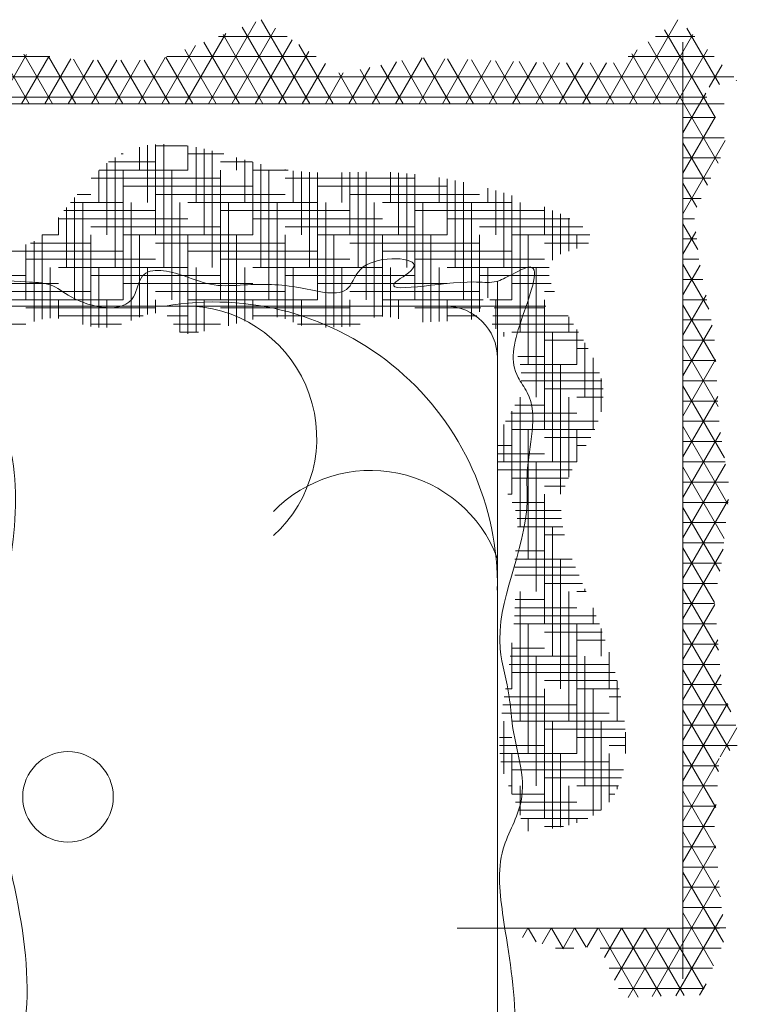
# Model space of a CAD drawing. Units: inches. Extents: x 3731 to 4318, y 1310 to 2388.
# Tile 38 of 57: x 3897 to 3942, y 2243 to 2305. Entities that reach past the tile are written whole.
import ezdxf

# ---------------------------------------------------------------- set-up
doc = ezdxf.new("R2010")
doc.units = ezdxf.units.IN
doc.layers.add('A-FURN', color=8, linetype='Continuous', lineweight=13)

# ---------------------------------------------------------------- blocks, each defined once
blk = doc.blocks.new('A$C200C7901')
for p, q in [((2.3121, 1.6596), (2.3121, 0.0201)), ((2, 0.2957), (2, 1.2957)), ((2.0224, 0.9977), (2.0224, 1.1977)), ((2.0224, 0.9977), (2.0224, 1.1977)), ((1.9974, 0.5977), (1.9974, 0.7977)), ((1.9974, 0.5977), (1.9974, 0.7977)), ((2.0724, 0.5977), (2.0724, 0.7977)), ((2.0724, 0.5977), (2.0724, 0.7977)), ((2.1474, 0.5977), (2.1474, 0.7977)), ((2.1474, 0.5977), (2.1474, 0.7977)), ((1.9849, 0.5477), (1.9849, 0.7477)), ((1.9849, 0.5477), (1.9849, 0.7477)), ((2.0599, 0.5477), (2.0599, 0.7477)), ((2.0599, 0.5477), (2.0599, 0.7477)), ((2.1349, 0.5477), (2.1349, 0.7477)), ((2.1349, 0.5477), (2.1349, 0.7477)), ((1.0407, 0.0275), (1.0407, 0.4323)), ((0.4061, 0.3703), (2.0386, 0.3703)), ((2.4073, 0.0839), (0.9625, 0.0839))]:
    blk.add_line(p, q)
at = {"linetype": 'ByBlock'}
for p, q in [((2.3224, 0.0468), (2.3224, 1.6627)), ((2.3224, 0.0468), (2.3224, 1.6627)), ((2.3537, 0.0056), (2.3537, 1.634)), ((2.3537, 0.0056), (2.3537, 1.634)), ((1.9724, 1.0977), (1.9724, 1.2927)), ((1.9724, 1.0977), (1.9724, 1.2927)), ((2.0474, 1.0977), (2.0474, 1.2977)), ((2.0474, 1.0977), (2.0474, 1.2977)), ((2.3849, 1.0607), (2.3849, 1.3013)), ((2.3849, 1.0607), (2.3849, 1.3013)), ((2.0349, 1.0477), (2.0349, 1.2477)), ((2.0349, 1.0477), (2.0349, 1.2477)), ((2.0099, 0.9477), (2.0099, 1.1477)), ((2.0099, 0.9477), (2.0099, 1.1477)), ((2.0849, 0.9477), (2.0849, 1.1477)), ((2.0849, 0.9477), (2.0849, 1.1477)), ((2.3121, 1.1408), (2.3884, 1.0967)), ((2.3121, 1.1408), (2.3884, 1.0967)), ((2.3121, 1.0928), (2.3915, 1.1386)), ((2.3121, 1.0928), (2.3915, 1.1386)), ((1.9974, 0.8977), (1.9974, 1.0977)), ((1.9974, 0.8977), (1.9974, 1.0977)), ((2.0099, 1.0977), (2.095, 1.0977)), ((2.0099, 1.0977), (2.095, 1.0977)), ((2.0724, 0.8977), (2.0724, 1.0977)), ((2.0724, 0.8977), (2.0724, 1.0977)), ((2.3121, 1.1047), (2.3851, 1.0625)), ((2.3121, 1.1047), (2.3851, 1.0625)), ((2.3121, 1.0567), (2.3887, 1.1009)), ((2.3121, 1.0567), (2.3887, 1.1009)), ((1.9763, 1.0852), (2.1005, 1.0852)), ((1.9763, 1.0852), (2.1005, 1.0852)), ((2.0974, 0.9977), (2.0974, 1.0909)), ((2.0974, 0.9977), (2.0974, 1.0909)), ((1.9799, 1.0727), (2.1099, 1.0727)), ((1.9799, 1.0727), (2.1099, 1.0727)), ((2.1099, 1.0477), (2.1099, 1.0729)), ((2.1099, 1.0477), (2.1099, 1.0729)), ((2.3121, 1.0686), (2.3813, 1.0286)), ((2.3121, 1.0686), (2.3813, 1.0286)), ((1.9815, 1.0602), (2.0599, 1.0602)), ((1.9815, 1.0602), (2.0599, 1.0602)), ((2.3121, 1.0206), (2.3851, 1.0628)), ((2.3121, 1.0206), (2.3851, 1.0628)), ((1.981, 1.0477), (2.0099, 1.0477)), ((1.981, 1.0477), (2.0099, 1.0477)), ((1.9849, 0.9171), (1.9849, 1.0477)), ((1.9849, 0.9171), (1.9849, 1.0477)), ((2.0599, 0.8477), (2.0599, 1.0477)), ((2.0599, 0.8477), (2.0599, 1.0477)), ((2.0599, 1.0352), (2.1523, 1.0352)), ((2.0599, 1.0352), (2.1523, 1.0352)), ((2.1099, 1.0477), (2.137, 1.0477)), ((2.1099, 1.0477), (2.137, 1.0477)), ((2.1349, 0.8477), (2.1349, 1.0477)), ((2.1349, 0.8477), (2.1349, 1.0477)), ((2.1474, 0.8977), (2.1474, 1.0391)), ((2.1474, 0.8977), (2.1474, 1.0391)), ((2.0099, 1.0227), (2.1678, 1.0227)), ((2.0099, 1.0227), (2.1678, 1.0227)), ((2.1599, 0.9477), (2.1599, 1.029)), ((2.1599, 0.9477), (2.1599, 1.029)), ((2.1724, 0.9977), (2.1724, 1.0189)), ((2.1724, 0.9977), (2.1724, 1.0189)), ((2.3121, 1.0325), (2.3795, 0.9936)), ((2.3121, 1.0325), (2.3795, 0.9936)), ((2.3121, 0.9846), (2.3809, 1.0242)), ((2.3121, 0.9846), (2.3809, 1.0242)), ((1.9718, 1.0102), (2.1599, 1.0102)), ((1.9718, 1.0102), (2.1599, 1.0102)), ((1.9688, 0.9977), (2.1099, 0.9977)), ((1.9688, 0.9977), (2.1099, 0.9977)), ((1.9724, 0.9504), (1.9724, 0.9977)), ((1.9724, 0.9504), (1.9724, 0.9977)), ((2.0474, 0.7977), (2.0474, 0.9977)), ((2.0474, 0.7977), (2.0474, 0.9977)), ((2.1224, 0.7977), (2.1224, 0.9977)), ((2.1224, 0.7977), (2.1224, 0.9977)), ((2.1974, 0.7977), (2.1974, 0.9972)), ((2.1974, 0.7977), (2.1974, 0.9972)), ((2.3121, 0.9964), (2.3795, 0.9575)), ((2.3121, 0.9964), (2.3795, 0.9575)), ((2.3121, 0.9485), (2.3795, 0.9874)), ((2.3121, 0.9485), (2.3795, 0.9874)), ((1.9671, 0.9852), (2.0599, 0.9852)), ((1.9671, 0.9852), (2.0599, 0.9852)), ((1.9672, 0.9727), (2.0099, 0.9727)), ((1.9672, 0.9727), (2.0099, 0.9727)), ((2.1099, 0.9727), (2.2204, 0.9727)), ((2.1099, 0.9727), (2.2204, 0.9727)), ((2.1599, 0.9852), (2.2095, 0.9852)), ((2.1599, 0.9852), (2.2095, 0.9852)), ((2.2099, 0.8477), (2.2099, 0.9848)), ((2.2099, 0.8477), (2.2099, 0.9848)), ((2.0599, 0.9602), (2.2294, 0.9602)), ((2.0599, 0.9602), (2.2294, 0.9602)), ((2.2224, 0.8977), (2.2224, 0.9702)), ((2.2224, 0.8977), (2.2224, 0.9702)), ((2.3121, 0.9603), (2.3795, 0.9215)), ((2.3121, 0.9603), (2.3795, 0.9215)), ((2.0099, 0.9477), (2.2099, 0.9477)), ((2.0099, 0.9477), (2.2099, 0.9477)), ((2.0349, 0.7477), (2.0349, 0.9477)), ((2.0349, 0.7477), (2.0349, 0.9477)), ((2.1099, 0.7477), (2.1099, 0.9477)), ((2.1099, 0.7477), (2.1099, 0.9477)), ((2.1849, 0.7477), (2.1849, 0.9477)), ((2.1849, 0.7477), (2.1849, 0.9477)), ((2.2349, 0.9477), (2.2349, 0.9506)), ((2.2349, 0.9477), (2.2349, 0.9506)), ((2.3121, 0.9124), (2.3795, 0.9513)), ((2.3121, 0.9124), (2.3795, 0.9513)), ((1.9781, 0.9352), (2.1599, 0.9352)), ((1.9781, 0.9352), (2.1599, 0.9352)), ((1.9829, 0.9227), (2.1099, 0.9227)), ((1.9829, 0.9227), (2.1099, 0.9227)), ((2.2099, 0.9227), (2.2455, 0.9227)), ((2.2099, 0.9227), (2.2455, 0.9227)), ((2.3121, 0.9243), (2.3838, 0.8829)), ((2.3121, 0.9243), (2.3838, 0.8829)), ((2.3121, 0.8763), (2.3795, 0.9152)), ((2.3121, 0.8763), (2.3795, 0.9152)), ((1.9871, 0.9102), (2.0599, 0.9102)), ((1.9871, 0.9102), (2.0599, 0.9102)), ((1.9894, 0.8977), (2.0099, 0.8977)), ((1.9894, 0.8977), (2.0099, 0.8977)), ((2.0224, 0.6977), (2.0224, 0.8977)), ((2.0224, 0.6977), (2.0224, 0.8977)), ((2.0974, 0.6977), (2.0974, 0.8977)), ((2.0974, 0.6977), (2.0974, 0.8977)), ((2.1099, 0.8977), (2.2496, 0.8977)), ((2.1099, 0.8977), (2.2496, 0.8977)), ((2.1599, 0.9102), (2.2481, 0.9102)), ((2.1599, 0.9102), (2.2481, 0.9102)), ((2.1724, 0.6977), (2.1724, 0.8977)), ((2.1724, 0.6977), (2.1724, 0.8977)), ((2.2474, 0.8489), (2.2474, 0.8977)), ((2.2474, 0.8489), (2.2474, 0.8977)), ((2.0599, 0.8852), (2.2501, 0.8852)), ((2.0599, 0.8852), (2.2501, 0.8852)), ((2.3121, 0.8882), (2.4022, 0.8362)), ((2.3121, 0.8882), (2.4022, 0.8362)), ((2.3121, 0.8402), (2.3842, 0.8818)), ((2.3121, 0.8402), (2.3842, 0.8818)), ((1.9724, 0.7977), (1.9724, 0.8703)), ((1.9724, 0.7977), (1.9724, 0.8703)), ((1.9849, 0.8477), (1.9849, 0.88)), ((1.9849, 0.8477), (1.9849, 0.88)), ((2.0099, 0.8727), (2.2099, 0.8727)), ((2.0099, 0.8727), (2.2099, 0.8727)), ((2.3849, 0.6497), (2.3849, 0.8801)), ((2.3849, 0.6497), (2.3849, 0.8801)), ((1.9599, 0.8317), (1.9599, 0.8604)), ((1.9599, 0.8317), (1.9599, 0.8604)), ((1.9599, 0.8602), (2.1599, 0.8602)), ((1.9599, 0.8602), (2.1599, 0.8602)), ((2.3121, 0.8041), (2.3958, 0.8524)), ((2.3121, 0.8041), (2.3958, 0.8524)), ((2.3121, 0.8521), (2.4205, 0.7895)), ((2.3121, 0.8521), (2.4205, 0.7895)), ((1.9574, 0.8477), (2.1099, 0.8477)), ((1.9574, 0.8477), (2.1099, 0.8477)), ((2.0099, 0.6477), (2.0099, 0.8477)), ((2.0099, 0.6477), (2.0099, 0.8477)), ((2.0849, 0.6477), (2.0849, 0.8477)), ((2.0849, 0.6477), (2.0849, 0.8477)), ((2.1599, 0.6477), (2.1599, 0.8477)), ((2.1599, 0.6477), (2.1599, 0.8477)), ((2.2099, 0.8477), (2.2472, 0.8477)), ((2.2099, 0.8477), (2.2472, 0.8477)), ((2.2349, 0.7923), (2.2349, 0.8477)), ((2.2349, 0.7923), (2.2349, 0.8477)), ((1.9593, 0.8352), (2.0599, 0.8352)), ((1.9593, 0.8352), (2.0599, 0.8352)), ((1.9615, 0.8227), (2.0099, 0.8227)), ((1.9615, 0.8227), (2.0099, 0.8227)), ((2.1099, 0.8227), (2.2425, 0.8227)), ((2.1099, 0.8227), (2.2425, 0.8227)), ((2.1599, 0.8352), (2.2451, 0.8352)), ((2.1599, 0.8352), (2.2451, 0.8352)), ((2.3121, 0.7681), (2.4073, 0.823)), ((2.3121, 0.7681), (2.4073, 0.823)), ((2.0599, 0.8102), (2.2396, 0.8102)), ((2.0599, 0.8102), (2.2396, 0.8102)), ((2.3121, 0.816), (2.4384, 0.7431)), ((2.3121, 0.816), (2.4384, 0.7431)), ((2.0099, 0.7977), (2.2099, 0.7977)), ((2.0099, 0.7977), (2.2099, 0.7977)), ((2.2224, 0.7483), (2.2224, 0.7977)), ((2.2224, 0.7483), (2.2224, 0.7977)), ((2.3121, 0.732), (2.4189, 0.7936)), ((2.3121, 0.732), (2.4189, 0.7936)), ((2.4162, 0.6946), (2.4162, 0.8006)), ((2.4162, 0.6946), (2.4162, 0.8006)), ((1.9699, 0.7852), (2.1599, 0.7852)), ((1.9699, 0.7852), (2.1599, 0.7852)), ((2.3121, 0.7799), (2.4287, 0.7126)), ((2.3121, 0.7799), (2.4287, 0.7126)), ((1.9734, 0.7727), (2.1099, 0.7727)), ((1.9734, 0.7727), (2.1099, 0.7727)), ((1.9767, 0.7602), (2.0599, 0.7602)), ((1.9767, 0.7602), (2.0599, 0.7602)), ((2.1599, 0.7602), (2.2258, 0.7602)), ((2.1599, 0.7602), (2.2258, 0.7602)), ((2.2099, 0.7727), (2.2294, 0.7727)), ((2.2099, 0.7727), (2.2294, 0.7727)), ((2.3121, 0.6959), (2.4303, 0.7641)), ((2.3121, 0.6959), (2.4303, 0.7641)), ((1.9797, 0.7477), (2.0099, 0.7477)), ((1.9797, 0.7477), (2.0099, 0.7477)), ((2.1099, 0.7477), (2.2222, 0.7477)), ((2.1099, 0.7477), (2.2222, 0.7477)), ((2.2099, 0.6933), (2.2099, 0.7477)), ((2.2099, 0.6933), (2.2099, 0.7477)), ((2.0599, 0.7352), (2.2188, 0.7352)), ((2.0599, 0.7352), (2.2188, 0.7352)), ((2.3121, 0.7438), (2.4108, 0.6869)), ((2.3121, 0.7438), (2.4108, 0.6869)), ((2.3121, 0.6598), (2.4417, 0.7346)), ((2.3121, 0.6598), (2.4417, 0.7346)), ((2.0099, 0.7227), (2.2099, 0.7227)), ((2.0099, 0.7227), (2.2099, 0.7227)), ((1.9831, 0.7102), (2.1599, 0.7102)), ((1.9831, 0.7102), (2.1599, 0.7102)), ((2.3121, 0.7078), (2.3929, 0.6611)), ((2.3121, 0.7078), (2.3929, 0.6611)), ((1.9753, 0.6852), (2.0599, 0.6852)), ((1.9753, 0.6852), (2.0599, 0.6852)), ((1.9804, 0.6977), (2.1099, 0.6977)), ((1.9804, 0.6977), (2.1099, 0.6977)), ((2.0474, 0.4977), (2.0474, 0.6977)), ((2.0474, 0.4977), (2.0474, 0.6977)), ((2.1224, 0.4977), (2.1224, 0.6977)), ((2.1224, 0.4977), (2.1224, 0.6977)), ((2.1599, 0.6852), (2.2088, 0.6852)), ((2.1599, 0.6852), (2.2088, 0.6852)), ((2.1974, 0.4977), (2.1974, 0.6977)), ((2.1974, 0.4977), (2.1974, 0.6977)), ((2.2099, 0.6977), (2.2106, 0.6977)), ((2.2099, 0.6977), (2.2106, 0.6977)), ((1.97, 0.6727), (2.0099, 0.6727)), ((1.97, 0.6727), (2.0099, 0.6727)), ((1.9724, 0.5818), (1.9724, 0.6786)), ((1.9724, 0.5818), (1.9724, 0.6786)), ((2.1099, 0.6727), (2.2075, 0.6727)), ((2.1099, 0.6727), (2.2075, 0.6727)), ((2.3121, 0.6237), (2.4036, 0.6765)), ((2.3121, 0.6237), (2.4036, 0.6765)), ((2.3121, 0.6717), (2.3744, 0.6357)), ((2.3121, 0.6717), (2.3744, 0.6357)), ((2.0599, 0.6602), (2.2067, 0.6602)), ((2.0599, 0.6602), (2.2067, 0.6602)), ((2.0099, 0.6477), (2.2062, 0.6477)), ((2.0099, 0.6477), (2.2062, 0.6477)), ((2.0349, 0.4477), (2.0349, 0.6477)), ((2.0349, 0.4477), (2.0349, 0.6477)), ((2.1099, 0.4477), (2.1099, 0.6477)), ((2.1099, 0.4477), (2.1099, 0.6477)), ((2.1849, 0.4477), (2.1849, 0.6477)), ((2.1849, 0.4477), (2.1849, 0.6477)), ((1.9673, 0.6352), (2.1599, 0.6352)), ((1.9673, 0.6352), (2.1599, 0.6352)), ((2.3121, 0.6356), (2.3598, 0.6081)), ((2.3121, 0.6356), (2.3598, 0.6081)), ((1.9678, 0.6227), (2.1099, 0.6227)), ((1.9678, 0.6227), (2.1099, 0.6227)), ((1.9679, 0.6102), (2.0599, 0.6102)), ((1.9679, 0.6102), (2.0599, 0.6102)), ((2.1599, 0.6102), (2.2064, 0.6102)), ((2.1599, 0.6102), (2.2064, 0.6102)), ((2.3121, 0.5876), (2.3598, 0.6151)), ((2.3121, 0.5876), (2.3598, 0.6151)), ((1.9685, 0.5977), (2.0099, 0.5977)), ((1.9685, 0.5977), (2.0099, 0.5977)), ((2.0224, 0.3977), (2.0224, 0.5977)), ((2.0224, 0.3977), (2.0224, 0.5977)), ((2.0974, 0.3977), (2.0974, 0.5977)), ((2.0974, 0.3977), (2.0974, 0.5977)), ((2.1099, 0.5977), (2.2066, 0.5977)), ((2.1099, 0.5977), (2.2066, 0.5977)), ((2.1724, 0.3977), (2.1724, 0.5977)), ((2.1724, 0.3977), (2.1724, 0.5977)), ((2.3121, 0.5995), (2.3682, 0.5671)), ((2.3121, 0.5995), (2.3682, 0.5671)), ((2.0599, 0.5852), (2.2069, 0.5852)), ((2.0599, 0.5852), (2.2069, 0.5852)), ((2.3121, 0.5515), (2.365, 0.5821)), ((2.3121, 0.5515), (2.365, 0.5821)), ((2.0099, 0.5727), (2.207, 0.5727)), ((2.0099, 0.5727), (2.207, 0.5727)), ((2.3121, 0.5634), (2.3771, 0.5259)), ((2.3121, 0.5634), (2.3771, 0.5259)), ((1.9827, 0.5602), (2.1599, 0.5602)), ((1.9827, 0.5602), (2.1599, 0.5602)), ((1.9842, 0.5477), (2.1099, 0.5477)), ((1.9842, 0.5477), (2.1099, 0.5477)), ((2.0099, 0.3923), (2.0099, 0.5477)), ((2.0099, 0.3923), (2.0099, 0.5477)), ((2.0849, 0.3477), (2.0849, 0.5477)), ((2.0849, 0.3477), (2.0849, 0.5477)), ((2.1599, 0.3477), (2.1599, 0.5477)), ((2.1599, 0.3477), (2.1599, 0.5477)), ((2.3121, 0.5155), (2.3719, 0.55)), ((2.3121, 0.5155), (2.3719, 0.55)), ((1.9831, 0.5352), (2.0599, 0.5352)), ((1.9831, 0.5352), (2.0599, 0.5352)), ((2.1599, 0.5352), (2.2065, 0.5352)), ((2.1599, 0.5352), (2.2065, 0.5352)), ((1.9807, 0.5227), (2.0099, 0.5227)), ((1.9807, 0.5227), (2.0099, 0.5227)), ((2.1099, 0.5227), (2.2058, 0.5227)), ((2.1099, 0.5227), (2.2058, 0.5227)), ((2.3121, 0.5273), (2.383, 0.4864)), ((2.3121, 0.5273), (2.383, 0.4864)), ((2.3121, 0.4794), (2.3788, 0.5179)), ((2.3121, 0.4794), (2.3788, 0.5179)), ((2.0599, 0.5102), (2.2049, 0.5102)), ((2.0599, 0.5102), (2.2049, 0.5102)), ((1.9974, 0.3957), (1.9974, 0.4977)), ((1.9974, 0.3957), (1.9974, 0.4977)), ((2.0099, 0.4977), (2.2038, 0.4977)), ((2.0099, 0.4977), (2.2038, 0.4977)), ((2.0724, 0.2977), (2.0724, 0.4977)), ((2.0724, 0.2977), (2.0724, 0.4977)), ((2.1474, 0.2977), (2.1474, 0.4977)), ((2.1474, 0.2977), (2.1474, 0.4977)), ((2.3121, 0.4912), (2.3817, 0.4511)), ((2.3121, 0.4912), (2.3817, 0.4511)), ((1.9755, 0.4852), (2.1599, 0.4852)), ((1.9755, 0.4852), (2.1599, 0.4852)), ((1.9757, 0.4727), (2.1099, 0.4727)), ((1.9757, 0.4727), (2.1099, 0.4727)), ((2.3121, 0.4433), (2.383, 0.4842)), ((2.3121, 0.4433), (2.383, 0.4842)), ((1.9762, 0.4602), (2.0599, 0.4602)), ((1.9762, 0.4602), (2.0599, 0.4602)), ((2.1599, 0.4602), (2.1987, 0.4602)), ((2.1599, 0.4602), (2.1987, 0.4602)), ((1.9768, 0.4477), (2.0099, 0.4477)), ((1.9768, 0.4477), (2.0099, 0.4477)), ((1.9849, 0.402), (1.9849, 0.4477)), ((1.9849, 0.402), (1.9849, 0.4477)), ((2.0599, 0.2903), (2.0599, 0.4477)), ((2.0599, 0.2903), (2.0599, 0.4477)), ((2.1099, 0.4477), (2.1965, 0.4477)), ((2.1099, 0.4477), (2.1965, 0.4477)), ((2.1349, 0.2582), (2.1349, 0.4477)), ((2.1349, 0.2582), (2.1349, 0.4477)), ((2.3121, 0.4552), (2.3803, 0.4158)), ((2.3121, 0.4552), (2.3803, 0.4158)), ((2.3121, 0.4072), (2.3815, 0.4473)), ((2.3121, 0.4072), (2.3815, 0.4473)), ((2.0599, 0.4352), (2.194, 0.4352)), ((2.0599, 0.4352), (2.194, 0.4352)), ((1.9797, 0.4102), (2.1599, 0.4102)), ((1.9797, 0.4102), (2.1599, 0.4102)), ((2.0099, 0.4227), (2.1913, 0.4227)), ((2.0099, 0.4227), (2.1913, 0.4227)), ((2.3121, 0.4191), (2.3789, 0.3805)), ((2.3121, 0.4191), (2.3789, 0.3805)), ((2.3121, 0.3711), (2.3801, 0.4103)), ((2.3121, 0.3711), (2.3801, 0.4103)), ((1.9915, 0.3977), (2.1099, 0.3977)), ((1.9915, 0.3977), (2.1099, 0.3977)), ((2.0474, 0.2905), (2.0474, 0.3977)), ((2.0474, 0.2905), (2.0474, 0.3977)), ((2.1224, 0.2385), (2.1224, 0.3977)), ((2.1224, 0.2385), (2.1224, 0.3977)), ((2.0099, 0.3477), (2.0099, 0.382)), ((2.0099, 0.3477), (2.0099, 0.382)), ((2.0127, 0.3852), (2.0599, 0.3852)), ((2.0127, 0.3852), (2.0599, 0.3852)), ((2.1599, 0.3852), (2.1819, 0.3852)), ((2.1599, 0.3852), (2.1819, 0.3852)), ((2.3121, 0.383), (2.3775, 0.3452)), ((2.3121, 0.383), (2.3775, 0.3452)), ((1.2974, 0.1977), (1.2974, 0.3647)), ((1.2974, 0.1977), (1.2974, 0.3647)), ((1.3099, 0.2477), (1.3099, 0.3663)), ((1.3099, 0.2477), (1.3099, 0.3663)), ((1.3224, 0.2977), (1.3224, 0.3669)), ((1.3224, 0.2977), (1.3224, 0.3669)), ((1.3349, 0.3477), (1.3349, 0.3668)), ((1.3349, 0.3477), (1.3349, 0.3668)), ((1.7474, 0.2546), (1.7474, 0.3689)), ((1.7474, 0.2546), (1.7474, 0.3689)), ((1.7599, 0.2477), (1.7599, 0.3703)), ((1.7599, 0.2477), (1.7599, 0.3703)), ((1.7724, 0.2977), (1.7724, 0.3703)), ((1.7724, 0.2977), (1.7724, 0.3703)), ((1.7849, 0.3477), (1.7849, 0.3703)), ((1.7849, 0.3477), (1.7849, 0.3703)), ((1.9648, 0.3727), (2.0099, 0.3727)), ((1.9648, 0.3727), (2.0099, 0.3727)), ((1.9724, 0.253), (1.9724, 0.3785)), ((1.9724, 0.253), (1.9724, 0.3785)), ((1.9849, 0.2609), (1.9849, 0.3774)), ((1.9849, 0.2609), (1.9849, 0.3774)), ((1.9974, 0.2977), (1.9974, 0.3753)), ((1.9974, 0.2977), (1.9974, 0.3753)), ((2.1099, 0.3727), (2.1784, 0.3727)), ((2.1099, 0.3727), (2.1784, 0.3727)), ((2.3121, 0.335), (2.3786, 0.3734)), ((2.3121, 0.335), (2.3786, 0.3734)), ((1.2599, 0.3477), (1.2599, 0.3531)), ((1.2599, 0.3477), (1.2599, 0.3531)), ((1.2785, 0.3602), (1.3599, 0.3602)), ((1.2785, 0.3602), (1.3599, 0.3602)), ((1.3724, 0.1977), (1.3724, 0.3634)), ((1.3724, 0.1977), (1.3724, 0.3634)), ((1.3849, 0.2477), (1.3849, 0.3616)), ((1.3849, 0.2477), (1.3849, 0.3616)), ((1.3974, 0.2977), (1.3974, 0.3597)), ((1.3974, 0.2977), (1.3974, 0.3597)), ((1.4099, 0.3477), (1.4099, 0.3578)), ((1.4099, 0.3477), (1.4099, 0.3578)), ((1.4474, 0.1977), (1.4474, 0.3521)), ((1.4474, 0.1977), (1.4474, 0.3521)), ((1.4599, 0.2477), (1.4599, 0.3504)), ((1.4599, 0.2477), (1.4599, 0.3504)), ((1.7099, 0.3477), (1.7099, 0.3539)), ((1.7099, 0.3477), (1.7099, 0.3539)), ((1.7599, 0.3602), (1.8177, 0.3602)), ((1.7599, 0.3602), (1.8177, 0.3602)), ((1.8224, 0.2148), (1.8224, 0.3575)), ((1.8224, 0.2148), (1.8224, 0.3575)), ((1.8349, 0.2477), (1.8349, 0.3497)), ((1.8349, 0.2477), (1.8349, 0.3497)), ((1.9532, 0.3602), (1.9599, 0.3602)), ((1.9532, 0.3602), (1.9599, 0.3602)), ((2.0599, 0.3602), (2.1747, 0.3602)), ((2.0599, 0.3602), (2.1747, 0.3602)), ((1.2148, 0.3352), (1.2599, 0.3352)), ((1.2148, 0.3352), (1.2599, 0.3352)), ((1.2224, 0.2106), (1.2224, 0.3375)), ((1.2224, 0.2106), (1.2224, 0.3375)), ((1.2349, 0.2477), (1.2349, 0.3422)), ((1.2349, 0.2477), (1.2349, 0.3422)), ((1.2474, 0.2977), (1.2474, 0.3476)), ((1.2474, 0.2977), (1.2474, 0.3476)), ((1.2475, 0.3477), (1.3099, 0.3477)), ((1.2475, 0.3477), (1.3099, 0.3477)), ((1.2849, 0.1758), (1.2849, 0.3477)), ((1.2849, 0.1758), (1.2849, 0.3477)), ((1.3599, 0.1741), (1.3599, 0.3477)), ((1.3599, 0.1741), (1.3599, 0.3477)), ((1.3599, 0.3352), (1.5599, 0.3352)), ((1.3599, 0.3352), (1.5599, 0.3352)), ((1.4099, 0.3477), (1.4806, 0.3477)), ((1.4099, 0.3477), (1.4806, 0.3477)), ((1.4349, 0.1886), (1.4349, 0.3477)), ((1.4349, 0.1886), (1.4349, 0.3477)), ((1.4724, 0.2977), (1.4724, 0.3487)), ((1.4724, 0.2977), (1.4724, 0.3487)), ((1.5099, 0.2129), (1.5099, 0.3447)), ((1.5099, 0.2129), (1.5099, 0.3447)), ((1.5224, 0.2177), (1.5224, 0.3438)), ((1.5224, 0.2177), (1.5224, 0.3438)), ((1.5349, 0.2477), (1.5349, 0.3431)), ((1.5349, 0.2477), (1.5349, 0.3431)), ((1.5474, 0.2977), (1.5474, 0.3428)), ((1.5474, 0.2977), (1.5474, 0.3428)), ((1.5849, 0.2443), (1.5849, 0.3434)), ((1.5849, 0.2443), (1.5849, 0.3434)), ((1.5974, 0.2496), (1.5974, 0.3435)), ((1.5974, 0.2496), (1.5974, 0.3435)), ((1.6099, 0.2546), (1.6099, 0.3432)), ((1.6099, 0.2546), (1.6099, 0.3432)), ((1.6224, 0.2977), (1.6224, 0.3424)), ((1.6224, 0.2977), (1.6224, 0.3424)), ((1.6599, 0.2695), (1.6599, 0.3394)), ((1.6599, 0.2695), (1.6599, 0.3394)), ((1.6599, 0.3352), (1.8599, 0.3352)), ((1.6599, 0.3352), (1.8599, 0.3352)), ((1.6724, 0.2713), (1.6724, 0.3398)), ((1.6724, 0.2713), (1.6724, 0.3398)), ((1.6849, 0.272), (1.6849, 0.3422)), ((1.6849, 0.272), (1.6849, 0.3422)), ((1.6974, 0.2977), (1.6974, 0.3472)), ((1.6974, 0.2977), (1.6974, 0.3472)), ((1.7099, 0.3477), (1.8383, 0.3477)), ((1.7099, 0.3477), (1.8383, 0.3477)), ((1.7349, 0.2607), (1.7349, 0.3477)), ((1.7349, 0.2607), (1.7349, 0.3477)), ((1.8099, 0.2201), (1.8099, 0.3477)), ((1.8099, 0.2201), (1.8099, 0.3477)), ((1.8474, 0.2977), (1.8474, 0.3432)), ((1.8474, 0.2977), (1.8474, 0.3432)), ((1.9099, 0.2477), (1.9099, 0.3349)), ((1.9099, 0.2477), (1.9099, 0.3349)), ((1.9224, 0.2977), (1.9224, 0.3385)), ((1.9224, 0.2977), (1.9224, 0.3385)), ((1.9599, 0.2452), (1.9599, 0.3477)), ((1.9599, 0.2452), (1.9599, 0.3477)), ((1.9599, 0.3352), (2.1599, 0.3352)), ((1.9599, 0.3352), (2.1599, 0.3352)), ((2.0099, 0.3477), (2.1708, 0.3477)), ((2.0099, 0.3477), (2.1708, 0.3477)), ((2.0349, 0.2874), (2.0349, 0.3477)), ((2.0349, 0.2874), (2.0349, 0.3477)), ((2.1099, 0.2274), (2.1099, 0.3477)), ((2.1099, 0.2274), (2.1099, 0.3477)), ((2.3121, 0.3469), (2.3761, 0.31)), ((2.3121, 0.3469), (2.3761, 0.31)), ((2.3121, 0.299), (2.3772, 0.3365)), ((2.3121, 0.299), (2.3772, 0.3365)), ((1.0194, 0.3103), (1.0407, 0.3227)), ((1.0194, 0.3103), (1.0407, 0.3227)), ((1.0261, 0.3316), (1.0407, 0.3232)), ((1.0261, 0.3316), (1.0407, 0.3232)), ((1.1904, 0.3227), (1.2099, 0.3227)), ((1.1904, 0.3227), (1.2099, 0.3227)), ((1.2099, 0.2308), (1.2099, 0.334)), ((1.2099, 0.2308), (1.2099, 0.334)), ((1.3099, 0.3227), (1.5099, 0.3227)), ((1.3099, 0.3227), (1.5099, 0.3227)), ((1.6099, 0.3227), (1.8099, 0.3227)), ((1.6099, 0.3227), (1.8099, 0.3227)), ((1.8849, 0.2093), (1.8849, 0.3337)), ((1.8849, 0.2093), (1.8849, 0.3337)), ((1.8974, 0.2129), (1.8974, 0.3335)), ((1.8974, 0.2129), (1.8974, 0.3335)), ((1.9099, 0.3227), (2.1099, 0.3227)), ((1.9099, 0.3227), (2.1099, 0.3227)), ((1.2599, 0.3102), (1.4599, 0.3102)), ((1.2599, 0.3102), (1.4599, 0.3102)), ((1.5599, 0.3102), (1.7599, 0.3102)), ((1.5599, 0.3102), (1.7599, 0.3102)), ((1.8599, 0.3102), (2.0599, 0.3102)), ((1.8599, 0.3102), (2.0599, 0.3102)), ((2.3121, 0.3108), (2.3755, 0.2742)), ((2.3121, 0.3108), (2.3755, 0.2742)), ((1.0164, 0.3011), (1.0407, 0.2871)), ((1.0164, 0.3011), (1.0407, 0.2871)), ((1.1974, 0.2683), (1.1974, 0.2977)), ((1.1974, 0.2683), (1.1974, 0.2977)), ((1.2099, 0.2977), (1.4099, 0.2977)), ((1.2099, 0.2977), (1.4099, 0.2977)), ((1.2724, 0.1788), (1.2724, 0.2977)), ((1.2724, 0.1788), (1.2724, 0.2977)), ((1.3474, 0.173), (1.3474, 0.2977)), ((1.3474, 0.173), (1.3474, 0.2977)), ((1.4224, 0.1854), (1.4224, 0.2977)), ((1.4224, 0.1854), (1.4224, 0.2977)), ((1.4974, 0.2083), (1.4974, 0.2977)), ((1.4974, 0.2083), (1.4974, 0.2977)), ((1.5099, 0.2977), (1.7099, 0.2977)), ((1.5099, 0.2977), (1.7099, 0.2977)), ((1.5724, 0.2389), (1.5724, 0.2977)), ((1.5724, 0.2389), (1.5724, 0.2977)), ((1.6474, 0.2668), (1.6474, 0.2977)), ((1.6474, 0.2668), (1.6474, 0.2977)), ((1.7224, 0.2658), (1.7224, 0.2977)), ((1.7224, 0.2658), (1.7224, 0.2977)), ((1.7974, 0.2263), (1.7974, 0.2977)), ((1.7974, 0.2263), (1.7974, 0.2977)), ((1.8099, 0.2977), (2.0099, 0.2977)), ((1.8099, 0.2977), (2.0099, 0.2977)), ((1.8724, 0.2072), (1.8724, 0.2977)), ((1.8724, 0.2072), (1.8724, 0.2977)), ((1.9474, 0.2376), (1.9474, 0.2977)), ((1.9474, 0.2376), (1.9474, 0.2977)), ((2.0224, 0.2822), (2.0224, 0.2977)), ((2.0224, 0.2822), (2.0224, 0.2977)), ((2.0974, 0.2299), (2.0974, 0.2977)), ((2.0974, 0.2299), (2.0974, 0.2977)), ((2.1099, 0.2977), (2.153, 0.2977)), ((2.1099, 0.2977), (2.153, 0.2977)), ((2.3121, 0.2629), (2.3757, 0.2996)), ((2.3121, 0.2629), (2.3757, 0.2996)), ((1.0089, 0.2682), (1.0407, 0.2866)), ((1.0089, 0.2682), (1.0407, 0.2866)), ((1.0099, 0.2521), (1.0099, 0.2804)), ((1.0099, 0.2521), (1.0099, 0.2804)), ((1.1943, 0.2852), (1.3599, 0.2852)), ((1.1943, 0.2852), (1.3599, 0.2852)), ((1.4599, 0.2852), (1.6599, 0.2852)), ((1.4599, 0.2852), (1.6599, 0.2852)), ((1.7599, 0.2852), (1.9599, 0.2852)), ((1.7599, 0.2852), (1.9599, 0.2852)), ((2.0708, 0.2852), (2.1478, 0.2852)), ((2.0708, 0.2852), (2.1478, 0.2852)), ((2.3121, 0.2747), (2.3755, 0.2381)), ((2.3121, 0.2747), (2.3755, 0.2381)), ((1.0088, 0.2694), (1.0407, 0.251)), ((1.0088, 0.2694), (1.0407, 0.251)), ((1.1965, 0.2727), (1.3099, 0.2727)), ((1.1965, 0.2727), (1.3099, 0.2727)), ((1.1994, 0.2602), (1.2599, 0.2602)), ((1.1994, 0.2602), (1.2599, 0.2602)), ((1.3599, 0.2602), (1.5599, 0.2602)), ((1.3599, 0.2602), (1.5599, 0.2602)), ((1.4099, 0.2727), (1.6099, 0.2727)), ((1.4099, 0.2727), (1.6099, 0.2727)), ((1.7099, 0.2727), (1.9099, 0.2727)), ((1.7099, 0.2727), (1.9099, 0.2727)), ((1.7361, 0.2602), (1.8599, 0.2602)), ((1.7361, 0.2602), (1.8599, 0.2602)), ((1.9599, 0.2602), (1.9838, 0.2602)), ((1.9599, 0.2602), (1.9838, 0.2602)), ((2.08, 0.2727), (2.1422, 0.2727)), ((2.08, 0.2727), (2.1422, 0.2727)), ((2.0848, 0.2602), (2.1359, 0.2602)), ((2.0848, 0.2602), (2.1359, 0.2602)), ((2.3121, 0.2268), (2.3755, 0.2634)), ((2.3121, 0.2268), (2.3755, 0.2634)), ((1.0111, 0.2334), (1.0407, 0.2505)), ((1.0111, 0.2334), (1.0407, 0.2505)), ((1.2031, 0.2477), (1.2099, 0.2477)), ((1.2031, 0.2477), (1.2099, 0.2477)), ((1.2599, 0.1831), (1.2599, 0.2477)), ((1.2599, 0.1831), (1.2599, 0.2477)), ((1.3099, 0.2477), (1.5099, 0.2477)), ((1.3099, 0.2477), (1.5099, 0.2477)), ((1.3349, 0.1723), (1.3349, 0.2477)), ((1.3349, 0.1723), (1.3349, 0.2477)), ((1.4099, 0.1825), (1.4099, 0.2477)), ((1.4099, 0.1825), (1.4099, 0.2477)), ((1.4849, 0.2039), (1.4849, 0.2477)), ((1.4849, 0.2039), (1.4849, 0.2477)), ((1.5599, 0.2335), (1.5599, 0.2477)), ((1.5599, 0.2335), (1.5599, 0.2477)), ((1.7599, 0.2477), (1.8099, 0.2477)), ((1.7599, 0.2477), (1.8099, 0.2477)), ((1.7849, 0.2332), (1.7849, 0.2477)), ((1.7849, 0.2332), (1.7849, 0.2477)), ((1.8599, 0.2068), (1.8599, 0.2477)), ((1.8599, 0.2068), (1.8599, 0.2477)), ((1.9099, 0.2477), (1.9639, 0.2477)), ((1.9099, 0.2477), (1.9639, 0.2477)), ((1.9349, 0.2304), (1.9349, 0.2477)), ((1.9349, 0.2304), (1.9349, 0.2477)), ((2.0888, 0.2477), (2.1099, 0.2477)), ((2.0888, 0.2477), (2.1099, 0.2477)), ((1.0112, 0.232), (1.0407, 0.215)), ((1.0112, 0.232), (1.0407, 0.215)), ((1.2599, 0.2352), (1.4599, 0.2352)), ((1.2599, 0.2352), (1.4599, 0.2352)), ((1.5599, 0.2352), (1.5638, 0.2352)), ((1.5599, 0.2352), (1.5638, 0.2352)), ((1.8599, 0.2352), (1.9433, 0.2352)), ((1.8599, 0.2352), (1.9433, 0.2352)), ((2.3121, 0.2387), (2.3755, 0.202)), ((2.3121, 0.2387), (2.3755, 0.202)), ((0.9344, 0.153), (1.0407, 0.2144)), ((0.9344, 0.153), (1.0407, 0.2144)), ((1.2142, 0.2227), (1.4099, 0.2227)), ((1.2142, 0.2227), (1.4099, 0.2227)), ((1.5099, 0.2227), (1.5346, 0.2227)), ((1.5099, 0.2227), (1.5346, 0.2227)), ((1.8099, 0.2227), (1.9203, 0.2227)), ((1.8099, 0.2227), (1.9203, 0.2227)), ((2.3121, 0.1907), (2.3755, 0.2273)), ((2.3121, 0.1907), (2.3755, 0.2273)), ((0.9787, 0.0381), (0.9787, 0.1976)), ((0.9787, 0.0381), (0.9787, 0.1976)), ((0.9953, 0.2051), (1.0407, 0.1789)), ((0.9953, 0.2051), (1.0407, 0.1789)), ((1.0099, 0.0251), (1.0099, 0.2117)), ((1.0099, 0.0251), (1.0099, 0.2117)), ((1.2227, 0.2102), (1.3599, 0.2102)), ((1.2227, 0.2102), (1.3599, 0.2102)), ((1.2351, 0.1977), (1.3099, 0.1977)), ((1.2351, 0.1977), (1.3099, 0.1977)), ((1.2474, 0.1892), (1.2474, 0.1977)), ((1.2474, 0.1892), (1.2474, 0.1977)), ((1.3224, 0.1722), (1.3224, 0.1977)), ((1.3224, 0.1722), (1.3224, 0.1977)), ((1.3974, 0.1799), (1.3974, 0.1977)), ((1.3974, 0.1799), (1.3974, 0.1977)), ((1.4099, 0.1977), (1.4662, 0.1977)), ((1.4099, 0.1977), (1.4662, 0.1977)), ((1.4599, 0.2102), (1.5027, 0.2102)), ((1.4599, 0.2102), (1.5027, 0.2102)), ((1.8368, 0.2102), (1.8884, 0.2102)), ((1.8368, 0.2102), (1.8884, 0.2102)), ((2.3121, 0.2026), (2.3953, 0.1545)), ((2.3121, 0.2026), (2.3953, 0.1545)), ((0.9474, 0.0512), (0.9474, 0.1835)), ((0.9474, 0.0512), (0.9474, 0.1835)), ((0.9602, 0.1893), (1.0407, 0.1428)), ((0.9602, 0.1893), (1.0407, 0.1428)), ((1.2552, 0.1852), (1.2599, 0.1852)), ((1.2552, 0.1852), (1.2599, 0.1852)), ((1.3599, 0.1852), (1.4215, 0.1852)), ((1.3599, 0.1852), (1.4215, 0.1852)), ((2.3121, 0.1546), (2.3755, 0.1912)), ((2.3121, 0.1546), (2.3755, 0.1912)), ((0.9339, 0.1684), (1.0407, 0.1067)), ((0.9339, 0.1684), (1.0407, 0.1067)), ((0.9355, 0.1176), (1.0407, 0.1783)), ((0.9355, 0.1176), (1.0407, 0.1783)), ((1.3099, 0.1727), (1.3428, 0.1727)), ((1.3099, 0.1727), (1.3428, 0.1727)), ((2.3849, 0.0355), (2.3849, 0.1686)), ((2.3849, 0.0355), (2.3849, 0.1686)), ((2.3121, 0.1665), (2.4419, 0.0916)), ((2.3121, 0.1665), (2.4419, 0.0916)), ((2.3121, 0.1185), (2.3891, 0.163)), ((2.3121, 0.1185), (2.3891, 0.163)), ((0.9366, 0.0822), (1.0407, 0.1422)), ((0.9366, 0.0822), (1.0407, 0.1422)), ((2.2208, 0.0297), (2.4078, 0.1377)), ((2.2208, 0.0297), (2.4078, 0.1377)), ((0.935, 0.1316), (1.114, 0.0283)), ((0.935, 0.1316), (1.114, 0.0283)), ((2.3121, 0.1304), (2.4193, 0.0685)), ((2.3121, 0.1304), (2.4193, 0.0685)), ((2.4162, 0.0655), (2.4162, 0.1264)), ((2.4162, 0.0655), (2.4162, 0.1264)), ((2.2903, 0.0337), (2.4265, 0.1124)), ((2.2903, 0.0337), (2.4265, 0.1124)), ((0.9362, 0.0948), (1.0616, 0.0225)), ((0.9362, 0.0948), (1.0616, 0.0225)), ((0.9463, 0.0516), (1.0407, 0.1061)), ((0.9463, 0.0516), (1.0407, 0.1061)), ((2.3121, 0.0943), (2.3958, 0.046)), ((2.3121, 0.0943), (2.3958, 0.046)), ((0.9826, 0.0365), (1.0647, 0.0839)), ((0.9826, 0.0365), (1.0647, 0.0839)), ((1.0189, 0.0214), (1.1272, 0.0839)), ((1.0189, 0.0214), (1.1272, 0.0839)), ((1.0412, 0.0179), (1.0412, 0.0839)), ((1.0412, 0.0179), (1.0412, 0.0839)), ((1.0724, 0.0243), (1.0724, 0.0839)), ((1.0724, 0.0243), (1.0724, 0.0839)), ((1.0801, 0.0839), (1.1675, 0.0335)), ((1.0801, 0.0839), (1.1675, 0.0335)), ((1.0891, 0.0259), (1.1897, 0.0839)), ((1.0891, 0.0259), (1.1897, 0.0839)), ((1.1037, 0.0273), (1.1037, 0.0839)), ((1.1037, 0.0273), (1.1037, 0.0839)), ((1.1349, 0.0303), (1.1349, 0.0839)), ((1.1349, 0.0303), (1.1349, 0.0839)), ((1.1426, 0.0839), (1.2313, 0.0327)), ((1.1426, 0.0839), (1.2313, 0.0327)), ((1.1642, 0.0331), (1.2522, 0.0839)), ((1.1642, 0.0331), (1.2522, 0.0839)), ((1.1662, 0.0333), (1.1662, 0.0839)), ((1.1662, 0.0333), (1.1662, 0.0839)), ((1.1974, 0.0351), (1.1974, 0.0839)), ((1.1974, 0.0351), (1.1974, 0.0839)), ((1.2051, 0.0839), (1.3023, 0.0278)), ((1.2051, 0.0839), (1.3023, 0.0278)), ((1.2266, 0.033), (1.3147, 0.0839)), ((1.2266, 0.033), (1.3147, 0.0839)), ((1.2287, 0.0329), (1.2287, 0.0839)), ((1.2287, 0.0329), (1.2287, 0.0839)), ((1.2599, 0.0308), (1.2599, 0.0839)), ((1.2599, 0.0308), (1.2599, 0.0839)), ((1.2676, 0.0839), (1.3871, 0.015)), ((1.2676, 0.0839), (1.3871, 0.015)), ((1.2824, 0.0292), (1.3772, 0.0839)), ((1.2824, 0.0292), (1.3772, 0.0839)), ((1.2912, 0.0286), (1.2912, 0.0839)), ((1.2912, 0.0286), (1.2912, 0.0839)), ((1.3146, 0.0117), (1.4397, 0.0839)), ((1.3146, 0.0117), (1.4397, 0.0839)), ((1.3224, 0), (1.3224, 0.0839)), ((1.3224, 0), (1.3224, 0.0839)), ((1.3301, 0.0839), (1.4312, 0.0256)), ((1.3301, 0.0839), (1.4312, 0.0256)), ((1.3537, 0.0022), (1.3537, 0.0839)), ((1.3537, 0.0022), (1.3537, 0.0839)), ((1.3743, 0.0101), (1.5022, 0.0839)), ((1.3743, 0.0101), (1.5022, 0.0839)), ((1.3849, 0.0141), (1.3849, 0.0839)), ((1.3849, 0.0141), (1.3849, 0.0839)), ((1.3926, 0.0839), (1.4856, 0.0302)), ((1.3926, 0.0839), (1.4856, 0.0302)), ((1.4162, 0.0243), (1.4162, 0.0839)), ((1.4162, 0.0243), (1.4162, 0.0839)), ((1.4474, 0.027), (1.4474, 0.0839)), ((1.4474, 0.027), (1.4474, 0.0839)), ((1.4551, 0.0839), (1.54, 0.0349)), ((1.4551, 0.0839), (1.54, 0.0349)), ((1.4693, 0.0288), (1.5647, 0.0839)), ((1.4693, 0.0288), (1.5647, 0.0839)), ((1.4787, 0.0296), (1.4787, 0.0839)), ((1.4787, 0.0296), (1.4787, 0.0839)), ((1.5099, 0.0323), (1.5099, 0.0839)), ((1.5099, 0.0323), (1.5099, 0.0839)), ((1.5176, 0.0839), (1.6251, 0.0219)), ((1.5176, 0.0839), (1.6251, 0.0219)), ((1.5412, 0.035), (1.5412, 0.0839)), ((1.5412, 0.035), (1.5412, 0.0839)), ((1.5427, 0.0351), (1.6272, 0.0839)), ((1.5427, 0.0351), (1.6272, 0.0839)), ((1.5724, 0.0308), (1.5724, 0.0839)), ((1.5724, 0.0308), (1.5724, 0.0839)), ((1.5801, 0.0839), (1.7018, 0.0137)), ((1.5801, 0.0839), (1.7018, 0.0137)), ((1.5911, 0.027), (1.6897, 0.0839)), ((1.5911, 0.027), (1.6897, 0.0839)), ((1.6037, 0.0245), (1.6037, 0.0839)), ((1.6037, 0.0245), (1.6037, 0.0839)), ((1.6349, 0.0208), (1.6349, 0.0839)), ((1.6349, 0.0208), (1.6349, 0.0839)), ((1.6416, 0.0201), (1.7522, 0.0839)), ((1.6416, 0.0201), (1.7522, 0.0839)), ((1.6426, 0.0839), (1.7565, 0.0182)), ((1.6426, 0.0839), (1.7565, 0.0182)), ((1.6662, 0.0175), (1.6662, 0.0839)), ((1.6662, 0.0175), (1.6662, 0.0839)), ((1.6944, 0.0145), (1.8147, 0.0839)), ((1.6944, 0.0145), (1.8147, 0.0839)), ((1.6974, 0.0141), (1.6974, 0.0839)), ((1.6974, 0.0141), (1.6974, 0.0839)), ((1.7051, 0.0839), (1.8054, 0.026)), ((1.7051, 0.0839), (1.8054, 0.026)), ((1.7287, 0.0137), (1.7287, 0.0839)), ((1.7287, 0.0137), (1.7287, 0.0839)), ((1.7599, 0.0187), (1.7599, 0.0839)), ((1.7599, 0.0187), (1.7599, 0.0839)), ((1.7659, 0.0197), (1.8772, 0.0839)), ((1.7659, 0.0197), (1.8772, 0.0839)), ((1.7676, 0.0839), (1.8606, 0.0303)), ((1.7676, 0.0839), (1.8606, 0.0303)), ((1.7912, 0.0237), (1.7912, 0.0839)), ((1.7912, 0.0237), (1.7912, 0.0839)), ((1.8224, 0.0281), (1.8224, 0.0839)), ((1.8224, 0.0281), (1.8224, 0.0839)), ((1.8301, 0.0839), (1.9175, 0.0335)), ((1.8301, 0.0839), (1.9175, 0.0335)), ((1.8452, 0.0294), (1.9397, 0.0839)), ((1.8452, 0.0294), (1.9397, 0.0839)), ((1.8537, 0.0299), (1.8537, 0.0839)), ((1.8537, 0.0299), (1.8537, 0.0839)), ((1.8849, 0.0316), (1.8849, 0.0839)), ((1.8849, 0.0316), (1.8849, 0.0839)), ((1.8926, 0.0839), (1.9706, 0.0389)), ((1.8926, 0.0839), (1.9706, 0.0389)), ((1.9146, 0.0333), (2.0022, 0.0839)), ((1.9146, 0.0333), (2.0022, 0.0839)), ((1.9162, 0.0334), (1.9162, 0.0839)), ((1.9162, 0.0334), (1.9162, 0.0839)), ((1.9474, 0.0352), (1.9474, 0.0839)), ((1.9474, 0.0352), (1.9474, 0.0839)), ((1.9551, 0.0839), (2.017, 0.0482)), ((1.9551, 0.0839), (2.017, 0.0482)), ((1.9787, 0.0405), (1.9787, 0.0839)), ((1.9787, 0.0405), (1.9787, 0.0839)), ((1.9953, 0.0438), (2.0647, 0.0839)), ((1.9953, 0.0438), (2.0647, 0.0839)), ((2.0099, 0.0468), (2.0099, 0.0839)), ((2.0099, 0.0468), (2.0099, 0.0839)), ((2.0176, 0.0839), (2.0634, 0.0575)), ((2.0176, 0.0839), (2.0634, 0.0575)), ((2.0412, 0.053), (2.0412, 0.0839)), ((2.0412, 0.053), (2.0412, 0.0839)), ((2.0724, 0.0592), (2.0724, 0.0839)), ((2.0724, 0.0592), (2.0724, 0.0839)), ((2.0801, 0.0839), (2.1147, 0.0639)), ((2.0801, 0.0839), (2.1147, 0.0639)), ((2.0873, 0.0609), (2.1272, 0.0839)), ((2.0873, 0.0609), (2.1272, 0.0839)), ((2.1037, 0.0627), (2.1037, 0.0839)), ((2.1037, 0.0627), (2.1037, 0.0839)), ((2.1349, 0.0662), (2.1349, 0.0839)), ((2.1349, 0.0662), (2.1349, 0.0839)), ((2.1426, 0.0839), (2.2557, 0.0186)), ((2.1426, 0.0839), (2.2557, 0.0186)), ((2.1526, 0.0625), (2.1897, 0.0839)), ((2.1526, 0.0625), (2.1897, 0.0839)), ((2.1662, 0.056), (2.1662, 0.0839)), ((2.1662, 0.056), (2.1662, 0.0839)), ((2.1867, 0.0461), (2.2522, 0.0839)), ((2.1867, 0.0461), (2.2522, 0.0839)), ((2.1974, 0.041), (2.1974, 0.0839)), ((2.1974, 0.041), (2.1974, 0.0839)), ((2.2051, 0.0839), (2.2913, 0.0342)), ((2.2051, 0.0839), (2.2913, 0.0342)), ((2.2287, 0.0259), (2.2287, 0.0839)), ((2.2287, 0.0259), (2.2287, 0.0839)), ((2.2599, 0.0205), (2.2599, 0.0839)), ((2.2599, 0.0205), (2.2599, 0.0839)), ((2.2676, 0.0839), (2.3285, 0.0488)), ((2.2676, 0.0839), (2.3285, 0.0488)), ((2.2912, 0.0341), (2.2912, 0.0839)), ((2.2912, 0.0341), (2.2912, 0.0839)), ((2.3417, 0.0273), (2.429, 0.0777)), ((2.3417, 0.0273), (2.429, 0.0777)), ((0.9374, 0.0581), (0.9545, 0.0482)), ((0.9374, 0.0581), (0.9545, 0.0482)), ((2.338, 0.0433), (2.3723, 0.0235)), ((2.338, 0.0433), (2.3723, 0.0235)), ((1.3048, 0.0264), (1.3494, 0.0006)), ((1.3048, 0.0264), (1.3494, 0.0006)), ((2.3476, 0.0017), (2.3488, 0.001)), ((2.3476, 0.0017), (2.3488, 0.001))]:
    blk.add_line(p, q, dxfattribs=at)
blk.add_circle((1.2431, 1.0329), 0.0699)
for centre, radius, start, end in [((1.5693, 0.8075), 0.4372, 269.0679, 9.9322), ((1.7969, 0.8525), 0.2035, 222.1514, 356.4639), ((1.5372, 0.5659), 0.2094, 290.9415, 45.7647), ((1.92, 0.4503), 0.08, 270, 0)]:
    blk.add_arc(centre, radius, start, end)
blk.add_open_spline([(0.4856, 1.3429), (0.5504, 1.3182), (0.6715, 1.2721), (0.8374, 1.0498), (1.1164, 1.1183), (1.3878, 1.1816), (1.5888, 1.1102), (1.8403, 1.1127), (1.9415, 1.2178), (2.0032, 1.2819)], degree=3, knots=[0, 0, 0, 0, 205.411753, 383.654933, 772.067458, 921.644661, 1226.793228, 1388.983508, 1642.292305, 1642.292305, 1642.292305, 1642.292305])
blk.add_open_spline([(0.473, 1.2954), (0.4739, 1.2781), (0.4755, 1.2477), (0.5032, 1.2084), (0.4801, 1.1701), (0.4928, 1.1255), (0.4674, 1.0912), (0.4579, 1.0351), (0.501, 0.9724), (0.4311, 0.8832), (0.4902, 0.8637), (0.4843, 0.8288), (0.4774, 0.7906), (0.4625, 0.7457), (0.459, 0.6999), (0.4816, 0.6664), (0.4748, 0.625), (0.4791, 0.5889), (0.4533, 0.5528), (0.4738, 0.5004), (0.4658, 0.4502), (0.4696, 0.3946), (0.4189, 0.3935), (0.4493, 0.3684), (0.4694, 0.3857), (0.4922, 0.3576), (0.5297, 0.3262), (0.5917, 0.3353), (0.6454, 0.3754), (0.7083, 0.3741), (0.7643, 0.3328), (0.826, 0.346), (0.925, 0.3388), (1.0353, 0.3593), (1.1561, 0.3744), (1.2477, 0.3154), (1.3302, 0.3474), (1.4086, 0.3512), (1.5217, 0.3878), (1.6362, 0.3176), (1.7682, 0.3285), (1.8402, 0.3019), (1.9071, 0.3529), (1.9647, 0.3412), (2.0795, 0.2948), (2.0472, 0.3498), (2.0343, 0.3772), (2.0435, 0.43), (2.0109, 0.5782), (2.0746, 0.4643), (2.0805, 0.584), (2.0084, 0.5979), (2.0343, 0.6846), (2.0344, 0.746), (2.0293, 0.8096), (2.0489, 0.8545), (2.0652, 0.9218), (1.9842, 0.9297), (2.0007, 1.0162), (2.0367, 1.0585), (2.0367, 1.1102), (2.0457, 1.1647), (2.0226, 1.2084), (2.0234, 1.2306), (2.0236, 1.2352)], degree=3, knots=[0, 0, 0, 0, 51.660678, 90.967412, 128.902454, 170.303599, 219.852997, 247.834962, 336.321557, 429.35469, 458.821847, 477.222321, 524.135809, 581.038434, 617.839381, 657.146115, 693.947125, 740.178081, 760.753248, 820.731705, 885.133458, 928.777044, 953.563729, 976.574207, 995.553042, 1018.563482, 1064.584401, 1147.951297, 1174.787598, 1266.851571, 1308.018447, 1377.066427, 1441.511314, 1608.245014, 1714.11869, 1792.771707, 1913.247991, 1954.931389, 2029.864445, 2259.189419, 2305.221512, 2429.507982, 2456.344283, 2543.92595, 2627.925037, 2662.96218, 2687.736879, 2719.937755, 2839.540991, 2875.47895, 2953.681041, 2993.270313, 3066.872333, 3154.395764, 3200.397042, 3248.426375, 3312.828127, 3347.881398, 3444.484026, 3481.577522, 3518.665244, 3592.267265, 3644.719162, 3658.519501, 3658.519501, 3658.519501, 3658.519501], dxfattribs=at)

msp = doc.modelspace()

# ---------------------------------------------------------------- block references
at = {"layer": 'A-FURN', "xscale": 41.1071563136412, "yscale": 41.1071563136412, "zscale": 41.1071563136412, "rotation": 90}
msp.add_blockref('A$C200C7901', (3942.346, 2204.601), dxfattribs=at)

doc.saveas('drawing.dxf')
